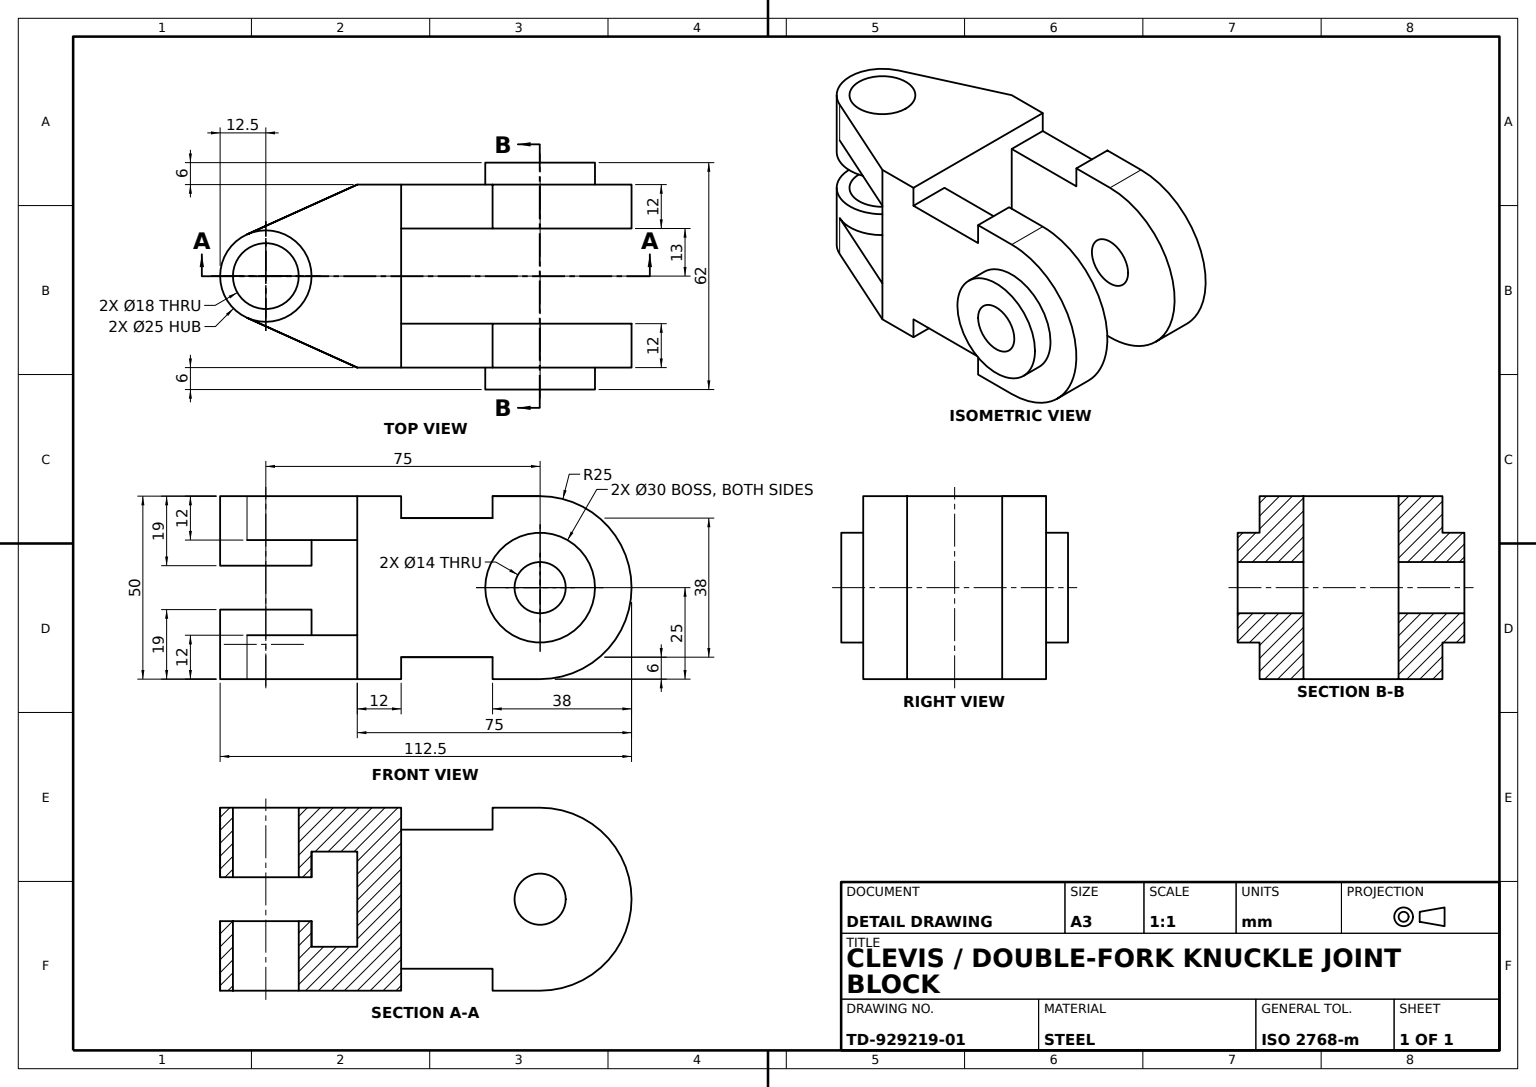
SolidWorks part; units mm, degrees
material "Plain Carbon Steel"
ref_plane "Front Plane" through (0, 0, 0) normal (0, 0, 1) x (1, 0, 0)
ref_plane "Top Plane" through (0, 0, 0) normal (0, 1, 0) x (1, 0, 0)
ref_plane "Right Plane" through (0, 0, 0) normal (1, 0, 0) x (0, 0, -1)
sketch "Main Body Side Profile Sketch" plane through (0, 0, 0) normal (1, 0, 0) x (0, 0, -1)
  line L0 (0, 0) -> (0, 50)
  line L1 (0, 50) -> (12, 50)
  line L2 (12, 50) -> (12, 44)
  line L3 (12, 44) -> (37, 44)
  line L4 (37, 44) -> (37, 50)
  line L5 (37, 50) -> (50, 50)
  line L7 (50, 0) -> (37, 0)
  line L8 (37, 0) -> (37, 6)
  line L9 (37, 6) -> (12, 6)
  line L10 (12, 6) -> (12, 0)
  line L11 (12, 0) -> (0, 0)
  arc A0 (50, 50) -> (50, 0) centre (50, 25) cw
  point P14 (75, 25)
  dimension "D10" = 25
  dimension "D1" = 50
  dimension "D2" = 38
  dimension "D3" = 25
  dimension "D4" = 6
  dimension "D5" = 12
  dimension "D6" = 13
  dimension "D7" = 75
  dimension "D8" = 50
  dimension "D9" = 12
  dimension "D11" = 50
extrude "Main Body" add sketch "Main Body Side Profile Sketch" along normal blind 12
sketch "Upper Plate Sketch" plane through (0, 0, 0) normal (0, 0, 1) x (1, 0, 0)
  line L1 (12, 50) -> (-38, 50)
  line L2 (12, 50) -> (12, 0)
  line L3 (12, 0) -> (-38, 0)
  line L4 (-38, 50) -> (-38, 0)
  dimension "D1" = 50
extrude "Upper Plate" add sketch "Upper Plate Sketch" against normal blind 12
sketch "Web Block Sketch" plane through (-38, 0, 0) normal (-1, 0, 0) x (0, 0, 1)
  line L0 (-12, 44) -> (-37, 44)
  line L1 (-37, 44) -> (-37, 50)
  line L2 (-37, 50) -> (-50, 50)
  line L3 (-12, 44) -> (-12, 6)
  line L4 (-12, 6) -> (-37, 6)
  line L5 (-37, 6) -> (-37, 0)
  line L6 (-37, 0) -> (-50, 0)
  arc A0 (-50, 50) -> (-50, 0) centre (-50, 25) ccw
  dimension "D1" = 25
extrude "Web Block" add sketch "Web Block Sketch" against normal blind 12
sketch "Pin Hub Boss A Sketch" plane through (12, 0, 0) normal (1, 0, 0) x (0, 0, -1)
  circle A0 centre (50, 25) radius 15
  circle A1 centre (50, 25) radius 7
  dimension "D1" = 30
  dimension "D2" = 14
extrude "Pin Hub Boss A Ø30" add sketch "Pin Hub Boss A Sketch" along normal blind 6
sketch "Pin Bore Sketch" plane through (12, 0, 0) normal (1, 0, 0) x (0, 0, -1)
  circle A0 centre (50, 25) radius 7
  dimension "D1" = 14
extrude "Pin Bore Ø14" cut sketch "Pin Bore Sketch" against normal blind 62
sketch "Pin Hub Boss B Sketch" plane through (-38, 0, 0) normal (-1, 0, 0) x (0, 0, 1)
  circle A0 centre (-50, 25) radius 15
  circle A1 centre (-50, 25) radius 7
  dimension "D1" = 30
  dimension "D2" = 14
extrude "Pin Hub Boss B Ø30" add sketch "Pin Hub Boss B Sketch" along normal blind 6
ref_plane "Plane1" through (0, 50, 0) normal (0, 1, 0) x (1, 0, 0)
sketch "Fork Lug Sketch" plane through (0, 50, 0) normal (0, 1, 0) x (1, 0, 0)
  line L0 (12, 0) -> (-38, 0) construction
  line L1 (-38, 0) -> (-24.393, -30.143)
  line L2 (-1.607, -30.143) -> (12, 0)
  line L3 (-38, 0) -> (12, 0)
  arc A0 (-24.393, -30.143) -> (-1.607, -30.143) centre (-13, -25) ccw
  point P4 (-13, 0)
  dimension "D1" = 25
  dimension "D3" = 25
  dimension "D2" = 25
extrude "Fork Lug" add sketch "Fork Lug Sketch" against normal blind 12
sketch "Fork Hub Sketch" plane through (0, 50, 0) normal (0, 1, 0) x (1, 0, 0)
  circle A0 centre (-13, -25) radius 12.5
  dimension "D1" = 25
extrude "Fork Hub Ø25" add sketch "Fork Hub Sketch" against normal blind 19
sketch "Fork Bore Sketch" plane through (0, 50, 0) normal (0, 1, 0) x (1, 0, 0)
  circle A0 centre (-13, -25) radius 9
  dimension "D1" = 18
extrude "Fork Bore Ø18" cut sketch "Fork Bore Sketch" against normal through all
sketch "Fork Filler Block Sketch" plane through (0, 0, 0) normal (0, -1, 0) x (1, 0, 0)
  line L0 (-38, 0) -> (-24.393, 30.143)
  line L1 (-1.607, 30.143) -> (12, 0)
  line L2 (12, 0) -> (-38, 0)
  circle A0 centre (-13, 25) radius 9
  circle A1 centre (-13, 25) radius 12.5
  line M3 (12, 0) -> (-38, 0)
  dimension "D1" = 25
  dimension "D2" = 18
extrude "Fork Filler Block" add sketch "Fork Filler Block Sketch" against normal blind 12 contours A1 L0 L1 M3 | A1 A0
sketch "Fork Spacer Ring Sketch" plane through (0, 12, 0) normal (0, 1, 0) x (1, 0, 0)
  circle A0 centre (-13, -25) radius 9
  circle A1 centre (-13, -25) radius 12.5
  dimension "D1" = 25
  dimension "D2" = 18
extrude "Fork Spacer Ring Ø25" add sketch "Fork Spacer Ring Sketch" along normal blind 7
